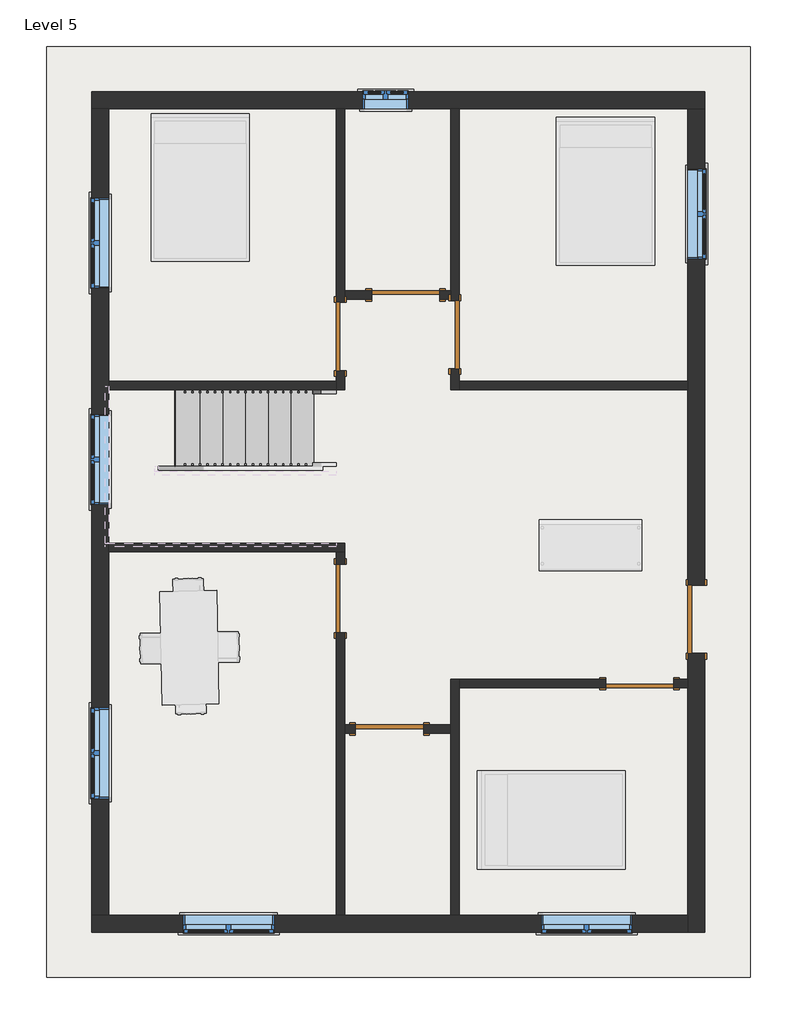
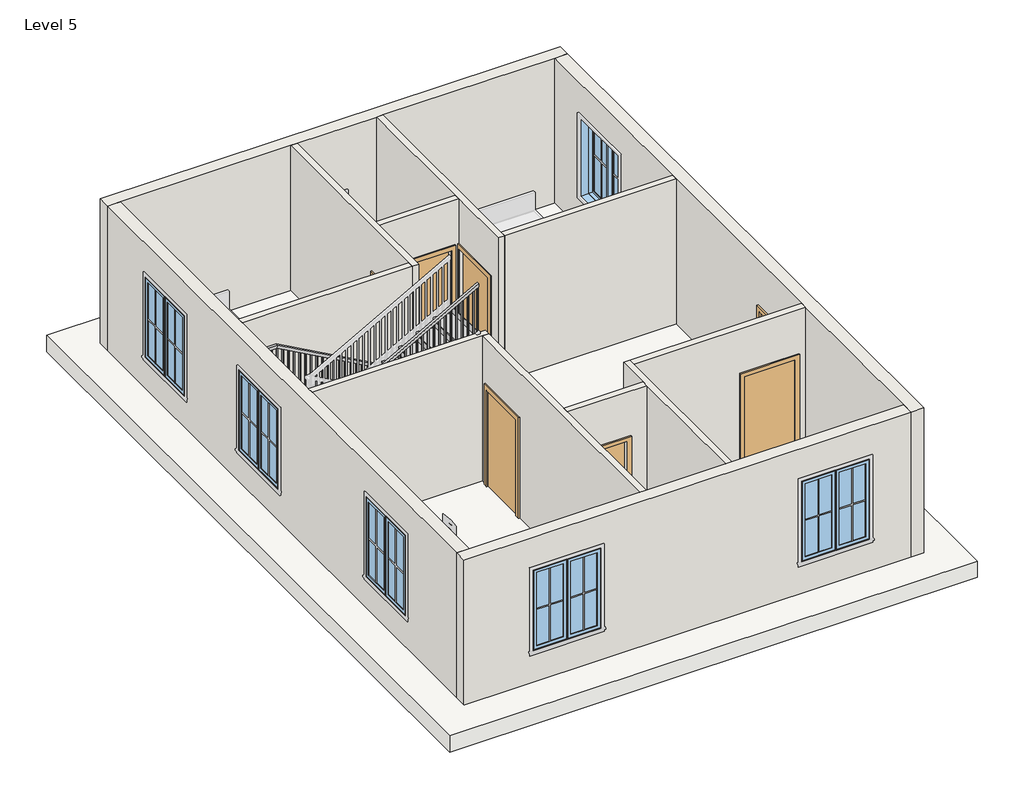
# One storey, part 1 of 2: 14 walls, 7 doors, 7 windows, 1 railing, 1 roof, 1 stair flight.
"""IFC4 building model written with IfcOpenShell, lengths in millimetres."""

from ifc_helpers import new_model, si_unit, frame, origin, place, context, project, spatial, polyline, outline, extrude, faceted_brep, transform, mapped, element, save
from components import door_e5f9f3c4, door_305aa2a5, door_a90ba1ad, stair_flight_99e02ff8, window_c417fced, window_8377141f

model = new_model("IFC4")

# Units and contexts
model_context = context("Model", 3, world=origin())
ifc_project = project(units=[si_unit("LENGTHUNIT", "METRE", prefix="MILLI")], contexts=[model_context])

# Site, building, storey
site = spatial("IfcSite", under=ifc_project)
building = spatial("IfcBuilding", under=site)
storey = spatial("IfcBuildingStorey", under=building, Name="Level 5", Elevation=12192.0)

# Doors
placement = place(None, origin())
door_shape = door_e5f9f3c4(model_context)
element("IfcDoor", 1, ObjectType="Single-Flush : 36\" x 84\"", at=placement, inside=storey, context=model_context, shape_type="MappedRepresentation", body=[
    mapped(door_shape, transform((5226.05, 11245.85, 12192.0), x_axis=(1.0, 0.0, 0.0), y_axis=(0.0, 1.0, 0.0), z_axis=(0.0, 0.0, 1.0))),
])
element("IfcDoor", 2, ObjectType="Single-Flush : 36\" x 84\"", at=placement, inside=storey, context=model_context, shape_type="MappedRepresentation", body=[
    mapped(door_shape, transform((5886.45, 10712.45, 12192.0), x_axis=(0.0, -1.0, 0.0), y_axis=(1.0, 0.0, 0.0), z_axis=(0.0, 0.0, 1.0))),
])
door_2_shape = door_305aa2a5(model_context)
element("IfcDoor", 3, ObjectType="Single-Flush : 36\" x 84\"", at=placement, inside=storey, context=model_context, shape_type="MappedRepresentation", body=[
    mapped(door_2_shape, transform((4349.75, 10687.05, 12192.0), x_axis=(0.0, -1.0, 0.0), y_axis=(1.0, 0.0, 0.0), z_axis=(0.0, 0.0, 1.0))),
])
element("IfcDoor", 4, ObjectType="Single-Flush : 36\" x 84\"", at=placement, inside=storey, context=model_context, shape_type="MappedRepresentation", body=[
    mapped(door_2_shape, transform((8369.3, 6026.15, 12192.0), x_axis=(1.0, 0.0, 0.0), y_axis=(0.0, 1.0, 0.0), z_axis=(0.0, 0.0, 1.0))),
])
element("IfcDoor", 5, ObjectType="Single-Flush : 36\" x 84\"", at=placement, inside=storey, context=model_context, shape_type="MappedRepresentation", body=[
    mapped(door_2_shape, transform((5010.15, 5416.55, 12192.0), x_axis=(-1.0, 0.0, 0.0), y_axis=(0.0, -1.0, 0.0), z_axis=(0.0, 0.0, 1.0))),
])
element("IfcDoor", 6, ObjectType="Single-Flush : 36\" x 84\"", at=placement, inside=storey, context=model_context, shape_type="MappedRepresentation", body=[
    mapped(door_2_shape, transform((4349.75, 7169.15, 12192.0), x_axis=(0.0, -1.0, 0.0), y_axis=(1.0, 0.0, 0.0), z_axis=(0.0, 0.0, 1.0))),
])
door_3_shape = door_a90ba1ad(model_context)
element("IfcDoor", 7, ObjectType="Single-Flush : 36\" x 84\"", at=placement, inside=storey, context=model_context, shape_type="MappedRepresentation", body=[
    mapped(door_3_shape, transform((9131.3, 6889.75, 12192.0), x_axis=(0.0, -1.0, 0.0), y_axis=(1.0, 0.0, 0.0), z_axis=(0.0, 0.0, 1.0))),
])

# Railing
element("IfcRailing", 8, ObjectType="Handrail - Rectangular", at=placement, inside=storey, context=model_context, shape_type="SolidModel", body=[
    faceted_brep([(4295.1355783, 9918.7, 13275.7333333), (4295.1355783, 9918.7, 13217.620221), (4295.1355783, 9969.5, 13217.620221), (4295.1355783, 9969.5, 13275.7333333), (1856.7355783, 9918.7, 14630.4), (1843.5719761, 9918.7, 14579.6), (1843.5719761, 9969.5, 14579.6), (1856.7355783, 9969.5, 14630.4), (1295.4, 9918.7, 14630.4), (1295.4, 9918.7, 14579.6), (1244.6, 9969.5, 14579.6), (1244.6, 9969.5, 14630.4), (1295.4, 7962.9, 14630.4), (1295.4, 7962.9, 14579.6), (1244.6, 7912.1, 14579.6), (1244.6, 7912.1, 14630.4), (1551.9355783, 7962.9, 14630.4), (1565.0991806, 7962.9, 14579.6), (1565.0991806, 7912.1, 14579.6), (1551.9355783, 7912.1, 14630.4), (4295.1355783, 7962.9, 16154.4), (4295.1355783, 7912.1, 16154.4), (4295.1355783, 7912.1, 16096.2868876), (4295.1355783, 7962.9, 16096.2868876)], [[[0, 1, 2, 3]], [[1, 0, 4, 5]], [[2, 1, 5, 6]], [[3, 2, 6, 7]], [[0, 3, 7, 4]], [[5, 4, 8, 9]], [[6, 5, 9, 10]], [[7, 6, 10, 11]], [[4, 7, 11, 8]], [[9, 8, 12, 13]], [[10, 9, 13, 14]], [[11, 10, 14, 15]], [[8, 11, 15, 12]], [[13, 12, 16, 17]], [[14, 13, 17, 18]], [[15, 14, 18, 19]], [[12, 15, 19, 16]], [[20, 21, 22, 23]], [[17, 16, 20, 23]], [[18, 17, 23, 22]], [[19, 18, 22, 21]], [[16, 19, 21, 20]]]),
    extrude(outline(polyline([(16057.8365664, 4225.925), (16047.253233, 4206.875), (15070.6666667, 4206.875), (15070.6666667, 4225.925), (16057.8365664, 4225.925)])), frame((0.0, 7927.975, 0.0), z_axis=(0.0, 1.0, 0.0), x_axis=(0.0, 0.0, 1.0)), (0.0, 0.0, 1.0), 19.05),
    extrude(outline(polyline([(16001.3921219, 4124.325), (15990.8087886, 4105.275), (15070.6666667, 4105.275), (15070.6666667, 4124.325), (16001.3921219, 4124.325)])), frame((0.0, 7927.975, 0.0), z_axis=(0.0, 1.0, 0.0), x_axis=(0.0, 0.0, 1.0)), (0.0, 0.0, 1.0), 19.05),
    extrude(outline(polyline([(15944.9476775, 4022.725), (15934.3643441, 4003.675), (15070.6666667, 4003.675), (15070.6666667, 4022.725), (15944.9476775, 4022.725)])), frame((0.0, 7927.975, 0.0), z_axis=(0.0, 1.0, 0.0), x_axis=(0.0, 0.0, 1.0)), (0.0, 0.0, 1.0), 19.05),
    extrude(outline(polyline([(15888.503233, 3921.125), (15877.9198997, 3902.075), (14901.3333333, 3902.075), (14901.3333333, 3921.125), (15888.503233, 3921.125)])), frame((0.0, 7927.975, 0.0), z_axis=(0.0, 1.0, 0.0), x_axis=(0.0, 0.0, 1.0)), (0.0, 0.0, 1.0), 19.05),
    extrude(outline(polyline([(15832.0587886, 3819.525), (15821.4754552, 3800.475), (14901.3333333, 3800.475), (14901.3333333, 3819.525), (15832.0587886, 3819.525)])), frame((0.0, 7927.975, 0.0), z_axis=(0.0, 1.0, 0.0), x_axis=(0.0, 0.0, 1.0)), (0.0, 0.0, 1.0), 19.05),
    extrude(outline(polyline([(15775.6143441, 3717.925), (15765.0310108, 3698.875), (14901.3333333, 3698.875), (14901.3333333, 3717.925), (15775.6143441, 3717.925)])), frame((0.0, 7927.975, 0.0), z_axis=(0.0, 1.0, 0.0), x_axis=(0.0, 0.0, 1.0)), (0.0, 0.0, 1.0), 19.05),
    extrude(outline(polyline([(15719.1698997, 3616.325), (15708.5865664, 3597.275), (14732.0, 3597.275), (14732.0, 3616.325), (15719.1698997, 3616.325)])), frame((0.0, 7927.975, 0.0), z_axis=(0.0, 1.0, 0.0), x_axis=(0.0, 0.0, 1.0)), (0.0, 0.0, 1.0), 19.05),
    extrude(outline(polyline([(15662.7254552, 3514.725), (15652.1421219, 3495.675), (14732.0, 3495.675), (14732.0, 3514.725), (15662.7254552, 3514.725)])), frame((0.0, 7927.975, 0.0), z_axis=(0.0, 1.0, 0.0), x_axis=(0.0, 0.0, 1.0)), (0.0, 0.0, 1.0), 19.05),
    extrude(outline(polyline([(15606.2810108, 3413.125), (15595.6976775, 3394.075), (14732.0, 3394.075), (14732.0, 3413.125), (15606.2810108, 3413.125)])), frame((0.0, 7927.975, 0.0), z_axis=(0.0, 1.0, 0.0), x_axis=(0.0, 0.0, 1.0)), (0.0, 0.0, 1.0), 19.05),
    extrude(outline(polyline([(15549.8365664, 3311.525), (15539.253233, 3292.475), (14562.6666667, 3292.475), (14562.6666667, 3311.525), (15549.8365664, 3311.525)])), frame((0.0, 7927.975, 0.0), z_axis=(0.0, 1.0, 0.0), x_axis=(0.0, 0.0, 1.0)), (0.0, 0.0, 1.0), 19.05),
    extrude(outline(polyline([(15493.3921219, 3209.925), (15482.8087886, 3190.875), (14562.6666667, 3190.875), (14562.6666667, 3209.925), (15493.3921219, 3209.925)])), frame((0.0, 7927.975, 0.0), z_axis=(0.0, 1.0, 0.0), x_axis=(0.0, 0.0, 1.0)), (0.0, 0.0, 1.0), 19.05),
    extrude(outline(polyline([(15436.9476775, 3108.325), (15426.3643441, 3089.275), (14562.6666667, 3089.275), (14562.6666667, 3108.325), (15436.9476775, 3108.325)])), frame((0.0, 7927.975, 0.0), z_axis=(0.0, 1.0, 0.0), x_axis=(0.0, 0.0, 1.0)), (0.0, 0.0, 1.0), 19.05),
    extrude(outline(polyline([(15380.503233, 3006.725), (15369.9198997, 2987.675), (14393.3333333, 2987.675), (14393.3333333, 3006.725), (15380.503233, 3006.725)])), frame((0.0, 7927.975, 0.0), z_axis=(0.0, 1.0, 0.0), x_axis=(0.0, 0.0, 1.0)), (0.0, 0.0, 1.0), 19.05),
    extrude(outline(polyline([(15324.0587886, 2905.125), (15313.4754552, 2886.075), (14393.3333333, 2886.075), (14393.3333333, 2905.125), (15324.0587886, 2905.125)])), frame((0.0, 7927.975, 0.0), z_axis=(0.0, 1.0, 0.0), x_axis=(0.0, 0.0, 1.0)), (0.0, 0.0, 1.0), 19.05),
    extrude(outline(polyline([(15267.6143441, 2803.525), (15257.0310108, 2784.475), (14393.3333333, 2784.475), (14393.3333333, 2803.525), (15267.6143441, 2803.525)])), frame((0.0, 7927.975, 0.0), z_axis=(0.0, 1.0, 0.0), x_axis=(0.0, 0.0, 1.0)), (0.0, 0.0, 1.0), 19.05),
    extrude(outline(polyline([(15211.1698997, 2701.925), (15200.5865664, 2682.875), (14224.0, 2682.875), (14224.0, 2701.925), (15211.1698997, 2701.925)])), frame((0.0, 7927.975, 0.0), z_axis=(0.0, 1.0, 0.0), x_axis=(0.0, 0.0, 1.0)), (0.0, 0.0, 1.0), 19.05),
    extrude(outline(polyline([(15154.7254552, 2600.325), (15144.1421219, 2581.275), (14224.0, 2581.275), (14224.0, 2600.325), (15154.7254552, 2600.325)])), frame((0.0, 7927.975, 0.0), z_axis=(0.0, 1.0, 0.0), x_axis=(0.0, 0.0, 1.0)), (0.0, 0.0, 1.0), 19.05),
    extrude(outline(polyline([(15098.2810108, 2498.725), (15087.6976775, 2479.675), (14224.0, 2479.675), (14224.0, 2498.725), (15098.2810108, 2498.725)])), frame((0.0, 7927.975, 0.0), z_axis=(0.0, 1.0, 0.0), x_axis=(0.0, 0.0, 1.0)), (0.0, 0.0, 1.0), 19.05),
    extrude(outline(polyline([(15041.8365664, 2397.125), (15031.253233, 2378.075), (14054.6666667, 2378.075), (14054.6666667, 2397.125), (15041.8365664, 2397.125)])), frame((0.0, 7927.975, 0.0), z_axis=(0.0, 1.0, 0.0), x_axis=(0.0, 0.0, 1.0)), (0.0, 0.0, 1.0), 19.05),
    extrude(outline(polyline([(14985.3921219, 2295.525), (14974.8087886, 2276.475), (14054.6666667, 2276.475), (14054.6666667, 2295.525), (14985.3921219, 2295.525)])), frame((0.0, 7927.975, 0.0), z_axis=(0.0, 1.0, 0.0), x_axis=(0.0, 0.0, 1.0)), (0.0, 0.0, 1.0), 19.05),
    extrude(outline(polyline([(14928.9476775, 2193.925), (14918.3643441, 2174.875), (14054.6666667, 2174.875), (14054.6666667, 2193.925), (14928.9476775, 2193.925)])), frame((0.0, 7927.975, 0.0), z_axis=(0.0, 1.0, 0.0), x_axis=(0.0, 0.0, 1.0)), (0.0, 0.0, 1.0), 19.05),
    extrude(outline(polyline([(14872.503233, 2092.325), (14861.9198997, 2073.275), (13885.3333333, 2073.275), (13885.3333333, 2092.325), (14872.503233, 2092.325)])), frame((0.0, 7927.975, 0.0), z_axis=(0.0, 1.0, 0.0), x_axis=(0.0, 0.0, 1.0)), (0.0, 0.0, 1.0), 19.05),
    extrude(outline(polyline([(14816.0587886, 1990.725), (14805.4754552, 1971.675), (13885.3333333, 1971.675), (13885.3333333, 1990.725), (14816.0587886, 1990.725)])), frame((0.0, 7927.975, 0.0), z_axis=(0.0, 1.0, 0.0), x_axis=(0.0, 0.0, 1.0)), (0.0, 0.0, 1.0), 19.05),
    extrude(outline(polyline([(14759.6143441, 1889.125), (14749.0310108, 1870.075), (13885.3333333, 1870.075), (13885.3333333, 1889.125), (14759.6143441, 1889.125)])), frame((0.0, 7927.975, 0.0), z_axis=(0.0, 1.0, 0.0), x_axis=(0.0, 0.0, 1.0)), (0.0, 0.0, 1.0), 19.05),
    extrude(outline(polyline([(14703.1698997, 1787.525), (14692.5865664, 1768.475), (13716.0, 1768.475), (13716.0, 1787.525), (14703.1698997, 1787.525)])), frame((0.0, 7927.975, 0.0), z_axis=(0.0, 1.0, 0.0), x_axis=(0.0, 0.0, 1.0)), (0.0, 0.0, 1.0), 19.05),
    extrude(outline(polyline([(14646.7254552, 1685.925), (14636.1421219, 1666.875), (13716.0, 1666.875), (13716.0, 1685.925), (14646.7254552, 1685.925)])), frame((0.0, 7927.975, 0.0), z_axis=(0.0, 1.0, 0.0), x_axis=(0.0, 0.0, 1.0)), (0.0, 0.0, 1.0), 19.05),
    extrude(outline(polyline([(14590.2810108, 1584.325), (14579.6976775, 1565.275), (13716.0, 1565.275), (13716.0, 1584.325), (14590.2810108, 1584.325)])), frame((0.0, 7927.975, 0.0), z_axis=(0.0, 1.0, 0.0), x_axis=(0.0, 0.0, 1.0)), (0.0, 0.0, 1.0), 19.05),
    extrude(outline(polyline([(1463.675, 7927.975), (1463.675, 7947.025), (1482.725, 7947.025), (1482.725, 7927.975), (1463.675, 7927.975)])), frame((0.0, 0.0, 13716.0), z_axis=(0.0, 0.0, 1.0), x_axis=(1.0, 0.0, 0.0)), (0.0, 0.0, 1.0), 863.6),
    extrude(outline(polyline([(1362.075, 7927.975), (1362.075, 7947.025), (1381.125, 7947.025), (1381.125, 7927.975), (1362.075, 7927.975)])), frame((0.0, 0.0, 13716.0), z_axis=(0.0, 0.0, 1.0), x_axis=(1.0, 0.0, 0.0)), (0.0, 0.0, 1.0), 863.6),
    extrude(outline(polyline([(1260.475, 8023.225), (1279.525, 8023.225), (1279.525, 8004.175), (1260.475, 8004.175), (1260.475, 8023.225)])), frame((0.0, 0.0, 13716.0), z_axis=(0.0, 0.0, 1.0), x_axis=(1.0, 0.0, 0.0)), (0.0, 0.0, 1.0), 863.6),
    extrude(outline(polyline([(1260.475, 8124.825), (1279.525, 8124.825), (1279.525, 8105.775), (1260.475, 8105.775), (1260.475, 8124.825)])), frame((0.0, 0.0, 13716.0), z_axis=(0.0, 0.0, 1.0), x_axis=(1.0, 0.0, 0.0)), (0.0, 0.0, 1.0), 863.6),
    extrude(outline(polyline([(1260.475, 8226.425), (1279.525, 8226.425), (1279.525, 8207.375), (1260.475, 8207.375), (1260.475, 8226.425)])), frame((0.0, 0.0, 13716.0), z_axis=(0.0, 0.0, 1.0), x_axis=(1.0, 0.0, 0.0)), (0.0, 0.0, 1.0), 863.6),
    extrude(outline(polyline([(1260.475, 8328.025), (1279.525, 8328.025), (1279.525, 8308.975), (1260.475, 8308.975), (1260.475, 8328.025)])), frame((0.0, 0.0, 13716.0), z_axis=(0.0, 0.0, 1.0), x_axis=(1.0, 0.0, 0.0)), (0.0, 0.0, 1.0), 863.6),
    extrude(outline(polyline([(1260.475, 8429.625), (1279.525, 8429.625), (1279.525, 8410.575), (1260.475, 8410.575), (1260.475, 8429.625)])), frame((0.0, 0.0, 13716.0), z_axis=(0.0, 0.0, 1.0), x_axis=(1.0, 0.0, 0.0)), (0.0, 0.0, 1.0), 863.6),
    extrude(outline(polyline([(1260.475, 8531.225), (1279.525, 8531.225), (1279.525, 8512.175), (1260.475, 8512.175), (1260.475, 8531.225)])), frame((0.0, 0.0, 13716.0), z_axis=(0.0, 0.0, 1.0), x_axis=(1.0, 0.0, 0.0)), (0.0, 0.0, 1.0), 863.6),
    extrude(outline(polyline([(1260.475, 8632.825), (1279.525, 8632.825), (1279.525, 8613.775), (1260.475, 8613.775), (1260.475, 8632.825)])), frame((0.0, 0.0, 13716.0), z_axis=(0.0, 0.0, 1.0), x_axis=(1.0, 0.0, 0.0)), (0.0, 0.0, 1.0), 863.6),
    extrude(outline(polyline([(1260.475, 8734.425), (1279.525, 8734.425), (1279.525, 8715.375), (1260.475, 8715.375), (1260.475, 8734.425)])), frame((0.0, 0.0, 13716.0), z_axis=(0.0, 0.0, 1.0), x_axis=(1.0, 0.0, 0.0)), (0.0, 0.0, 1.0), 863.6),
    extrude(outline(polyline([(1260.475, 8836.025), (1279.525, 8836.025), (1279.525, 8816.975), (1260.475, 8816.975), (1260.475, 8836.025)])), frame((0.0, 0.0, 13716.0), z_axis=(0.0, 0.0, 1.0), x_axis=(1.0, 0.0, 0.0)), (0.0, 0.0, 1.0), 863.6),
    extrude(outline(polyline([(1260.475, 8937.625), (1279.525, 8937.625), (1279.525, 8918.575), (1260.475, 8918.575), (1260.475, 8937.625)])), frame((0.0, 0.0, 13716.0), z_axis=(0.0, 0.0, 1.0), x_axis=(1.0, 0.0, 0.0)), (0.0, 0.0, 1.0), 863.6),
    extrude(outline(polyline([(1260.475, 9039.225), (1279.525, 9039.225), (1279.525, 9020.175), (1260.475, 9020.175), (1260.475, 9039.225)])), frame((0.0, 0.0, 13716.0), z_axis=(0.0, 0.0, 1.0), x_axis=(1.0, 0.0, 0.0)), (0.0, 0.0, 1.0), 863.6),
    extrude(outline(polyline([(1260.475, 9140.825), (1279.525, 9140.825), (1279.525, 9121.775), (1260.475, 9121.775), (1260.475, 9140.825)])), frame((0.0, 0.0, 13716.0), z_axis=(0.0, 0.0, 1.0), x_axis=(1.0, 0.0, 0.0)), (0.0, 0.0, 1.0), 863.6),
    extrude(outline(polyline([(1260.475, 9242.425), (1279.525, 9242.425), (1279.525, 9223.375), (1260.475, 9223.375), (1260.475, 9242.425)])), frame((0.0, 0.0, 13716.0), z_axis=(0.0, 0.0, 1.0), x_axis=(1.0, 0.0, 0.0)), (0.0, 0.0, 1.0), 863.6),
    extrude(outline(polyline([(1260.475, 9344.025), (1279.525, 9344.025), (1279.525, 9324.975), (1260.475, 9324.975), (1260.475, 9344.025)])), frame((0.0, 0.0, 13716.0), z_axis=(0.0, 0.0, 1.0), x_axis=(1.0, 0.0, 0.0)), (0.0, 0.0, 1.0), 863.6),
    extrude(outline(polyline([(1260.475, 9445.625), (1279.525, 9445.625), (1279.525, 9426.575), (1260.475, 9426.575), (1260.475, 9445.625)])), frame((0.0, 0.0, 13716.0), z_axis=(0.0, 0.0, 1.0), x_axis=(1.0, 0.0, 0.0)), (0.0, 0.0, 1.0), 863.6),
    extrude(outline(polyline([(1260.475, 9547.225), (1279.525, 9547.225), (1279.525, 9528.175), (1260.475, 9528.175), (1260.475, 9547.225)])), frame((0.0, 0.0, 13716.0), z_axis=(0.0, 0.0, 1.0), x_axis=(1.0, 0.0, 0.0)), (0.0, 0.0, 1.0), 863.6),
    extrude(outline(polyline([(1260.475, 9648.825), (1279.525, 9648.825), (1279.525, 9629.775), (1260.475, 9629.775), (1260.475, 9648.825)])), frame((0.0, 0.0, 13716.0), z_axis=(0.0, 0.0, 1.0), x_axis=(1.0, 0.0, 0.0)), (0.0, 0.0, 1.0), 863.6),
    extrude(outline(polyline([(1260.475, 9750.425), (1279.525, 9750.425), (1279.525, 9731.375), (1260.475, 9731.375), (1260.475, 9750.425)])), frame((0.0, 0.0, 13716.0), z_axis=(0.0, 0.0, 1.0), x_axis=(1.0, 0.0, 0.0)), (0.0, 0.0, 1.0), 863.6),
    extrude(outline(polyline([(1260.475, 9852.025), (1279.525, 9852.025), (1279.525, 9832.975), (1260.475, 9832.975), (1260.475, 9852.025)])), frame((0.0, 0.0, 13716.0), z_axis=(0.0, 0.0, 1.0), x_axis=(1.0, 0.0, 0.0)), (0.0, 0.0, 1.0), 863.6),
    extrude(outline(polyline([(1358.2605783, 9953.625), (1358.2605783, 9934.575), (1339.2105783, 9934.575), (1339.2105783, 9953.625), (1358.2605783, 9953.625)])), frame((0.0, 0.0, 13716.0), z_axis=(0.0, 0.0, 1.0), x_axis=(1.0, 0.0, 0.0)), (0.0, 0.0, 1.0), 863.6),
    extrude(outline(polyline([(1459.8605783, 9953.625), (1459.8605783, 9934.575), (1440.8105783, 9934.575), (1440.8105783, 9953.625), (1459.8605783, 9953.625)])), frame((0.0, 0.0, 13716.0), z_axis=(0.0, 0.0, 1.0), x_axis=(1.0, 0.0, 0.0)), (0.0, 0.0, 1.0), 863.6),
    extrude(outline(polyline([(1561.4605783, 9953.625), (1561.4605783, 9934.575), (1542.4105783, 9934.575), (1542.4105783, 9953.625), (1561.4605783, 9953.625)])), frame((0.0, 0.0, 13716.0), z_axis=(0.0, 0.0, 1.0), x_axis=(1.0, 0.0, 0.0)), (0.0, 0.0, 1.0), 863.6),
    extrude(outline(polyline([(1663.0605783, 9953.625), (1663.0605783, 9934.575), (1644.0105783, 9934.575), (1644.0105783, 9953.625), (1663.0605783, 9953.625)])), frame((0.0, 0.0, 13716.0), z_axis=(0.0, 0.0, 1.0), x_axis=(1.0, 0.0, 0.0)), (0.0, 0.0, 1.0), 863.6),
    extrude(outline(polyline([(1764.6605783, 9953.625), (1764.6605783, 9934.575), (1745.6105783, 9934.575), (1745.6105783, 9953.625), (1764.6605783, 9953.625)])), frame((0.0, 0.0, 13716.0), z_axis=(0.0, 0.0, 1.0), x_axis=(1.0, 0.0, 0.0)), (0.0, 0.0, 1.0), 863.6),
    extrude(outline(polyline([(14566.995221, 1866.2605783), (14577.5785543, 1847.2105783), (13716.0, 1847.2105783), (13716.0, 1866.2605783), (14566.995221, 1866.2605783)])), frame((0.0, 9934.575, 0.0), z_axis=(0.0, 1.0, 0.0), x_axis=(0.0, 0.0, 1.0)), (0.0, 0.0, 1.0), 19.05),
    extrude(outline(polyline([(14510.5507765, 1967.8605783), (14521.1341099, 1948.8105783), (13546.6666667, 1948.8105783), (13546.6666667, 1967.8605783), (14510.5507765, 1967.8605783)])), frame((0.0, 9934.575, 0.0), z_axis=(0.0, 1.0, 0.0), x_axis=(0.0, 0.0, 1.0)), (0.0, 0.0, 1.0), 19.05),
    extrude(outline(polyline([(14454.1063321, 2069.4605783), (14464.6896654, 2050.4105783), (13546.6666667, 2050.4105783), (13546.6666667, 2069.4605783), (14454.1063321, 2069.4605783)])), frame((0.0, 9934.575, 0.0), z_axis=(0.0, 1.0, 0.0), x_axis=(0.0, 0.0, 1.0)), (0.0, 0.0, 1.0), 19.05),
    extrude(outline(polyline([(14397.6618876, 2171.0605783), (14408.245221, 2152.0105783), (13546.6666667, 2152.0105783), (13546.6666667, 2171.0605783), (14397.6618876, 2171.0605783)])), frame((0.0, 9934.575, 0.0), z_axis=(0.0, 1.0, 0.0), x_axis=(0.0, 0.0, 1.0)), (0.0, 0.0, 1.0), 19.05),
    extrude(outline(polyline([(14341.2174432, 2272.6605783), (14351.8007765, 2253.6105783), (13377.3333333, 2253.6105783), (13377.3333333, 2272.6605783), (14341.2174432, 2272.6605783)])), frame((0.0, 9934.575, 0.0), z_axis=(0.0, 1.0, 0.0), x_axis=(0.0, 0.0, 1.0)), (0.0, 0.0, 1.0), 19.05),
    extrude(outline(polyline([(14284.7729988, 2374.2605783), (14295.3563321, 2355.2105783), (13377.3333333, 2355.2105783), (13377.3333333, 2374.2605783), (14284.7729988, 2374.2605783)])), frame((0.0, 9934.575, 0.0), z_axis=(0.0, 1.0, 0.0), x_axis=(0.0, 0.0, 1.0)), (0.0, 0.0, 1.0), 19.05),
    extrude(outline(polyline([(14228.3285543, 2475.8605783), (14238.9118876, 2456.8105783), (13377.3333333, 2456.8105783), (13377.3333333, 2475.8605783), (14228.3285543, 2475.8605783)])), frame((0.0, 9934.575, 0.0), z_axis=(0.0, 1.0, 0.0), x_axis=(0.0, 0.0, 1.0)), (0.0, 0.0, 1.0), 19.05),
    extrude(outline(polyline([(14171.8841099, 2577.4605783), (14182.4674432, 2558.4105783), (13208.0, 2558.4105783), (13208.0, 2577.4605783), (14171.8841099, 2577.4605783)])), frame((0.0, 9934.575, 0.0), z_axis=(0.0, 1.0, 0.0), x_axis=(0.0, 0.0, 1.0)), (0.0, 0.0, 1.0), 19.05),
    extrude(outline(polyline([(14115.4396654, 2679.0605783), (14126.0229988, 2660.0105783), (13208.0, 2660.0105783), (13208.0, 2679.0605783), (14115.4396654, 2679.0605783)])), frame((0.0, 9934.575, 0.0), z_axis=(0.0, 1.0, 0.0), x_axis=(0.0, 0.0, 1.0)), (0.0, 0.0, 1.0), 19.05),
    extrude(outline(polyline([(14058.995221, 2780.6605783), (14069.5785543, 2761.6105783), (13208.0, 2761.6105783), (13208.0, 2780.6605783), (14058.995221, 2780.6605783)])), frame((0.0, 9934.575, 0.0), z_axis=(0.0, 1.0, 0.0), x_axis=(0.0, 0.0, 1.0)), (0.0, 0.0, 1.0), 19.05),
    extrude(outline(polyline([(14002.5507765, 2882.2605783), (14013.1341099, 2863.2105783), (13038.6666667, 2863.2105783), (13038.6666667, 2882.2605783), (14002.5507765, 2882.2605783)])), frame((0.0, 9934.575, 0.0), z_axis=(0.0, 1.0, 0.0), x_axis=(0.0, 0.0, 1.0)), (0.0, 0.0, 1.0), 19.05),
    extrude(outline(polyline([(13946.1063321, 2983.8605783), (13956.6896654, 2964.8105783), (13038.6666667, 2964.8105783), (13038.6666667, 2983.8605783), (13946.1063321, 2983.8605783)])), frame((0.0, 9934.575, 0.0), z_axis=(0.0, 1.0, 0.0), x_axis=(0.0, 0.0, 1.0)), (0.0, 0.0, 1.0), 19.05),
    extrude(outline(polyline([(13889.6618876, 3085.4605783), (13900.245221, 3066.4105783), (13038.6666667, 3066.4105783), (13038.6666667, 3085.4605783), (13889.6618876, 3085.4605783)])), frame((0.0, 9934.575, 0.0), z_axis=(0.0, 1.0, 0.0), x_axis=(0.0, 0.0, 1.0)), (0.0, 0.0, 1.0), 19.05),
    extrude(outline(polyline([(13833.2174432, 3187.0605783), (13843.8007765, 3168.0105783), (12869.3333333, 3168.0105783), (12869.3333333, 3187.0605783), (13833.2174432, 3187.0605783)])), frame((0.0, 9934.575, 0.0), z_axis=(0.0, 1.0, 0.0), x_axis=(0.0, 0.0, 1.0)), (0.0, 0.0, 1.0), 19.05),
    extrude(outline(polyline([(13776.7729988, 3288.6605783), (13787.3563321, 3269.6105783), (12869.3333333, 3269.6105783), (12869.3333333, 3288.6605783), (13776.7729988, 3288.6605783)])), frame((0.0, 9934.575, 0.0), z_axis=(0.0, 1.0, 0.0), x_axis=(0.0, 0.0, 1.0)), (0.0, 0.0, 1.0), 19.05),
    extrude(outline(polyline([(13720.3285543, 3390.2605783), (13730.9118876, 3371.2105783), (12869.3333333, 3371.2105783), (12869.3333333, 3390.2605783), (13720.3285543, 3390.2605783)])), frame((0.0, 9934.575, 0.0), z_axis=(0.0, 1.0, 0.0), x_axis=(0.0, 0.0, 1.0)), (0.0, 0.0, 1.0), 19.05),
    extrude(outline(polyline([(13663.8841099, 3491.8605783), (13674.4674432, 3472.8105783), (12700.0, 3472.8105783), (12700.0, 3491.8605783), (13663.8841099, 3491.8605783)])), frame((0.0, 9934.575, 0.0), z_axis=(0.0, 1.0, 0.0), x_axis=(0.0, 0.0, 1.0)), (0.0, 0.0, 1.0), 19.05),
    extrude(outline(polyline([(13607.4396654, 3593.4605783), (13618.0229988, 3574.4105783), (12700.0, 3574.4105783), (12700.0, 3593.4605783), (13607.4396654, 3593.4605783)])), frame((0.0, 9934.575, 0.0), z_axis=(0.0, 1.0, 0.0), x_axis=(0.0, 0.0, 1.0)), (0.0, 0.0, 1.0), 19.05),
    extrude(outline(polyline([(13550.995221, 3695.0605783), (13561.5785543, 3676.0105783), (12700.0, 3676.0105783), (12700.0, 3695.0605783), (13550.995221, 3695.0605783)])), frame((0.0, 9934.575, 0.0), z_axis=(0.0, 1.0, 0.0), x_axis=(0.0, 0.0, 1.0)), (0.0, 0.0, 1.0), 19.05),
    extrude(outline(polyline([(13494.5507765, 3796.6605783), (13505.1341099, 3777.6105783), (12530.6666667, 3777.6105783), (12530.6666667, 3796.6605783), (13494.5507765, 3796.6605783)])), frame((0.0, 9934.575, 0.0), z_axis=(0.0, 1.0, 0.0), x_axis=(0.0, 0.0, 1.0)), (0.0, 0.0, 1.0), 19.05),
    extrude(outline(polyline([(13438.1063321, 3898.2605783), (13448.6896654, 3879.2105783), (12530.6666667, 3879.2105783), (12530.6666667, 3898.2605783), (13438.1063321, 3898.2605783)])), frame((0.0, 9934.575, 0.0), z_axis=(0.0, 1.0, 0.0), x_axis=(0.0, 0.0, 1.0)), (0.0, 0.0, 1.0), 19.05),
    extrude(outline(polyline([(13381.6618876, 3999.8605783), (13392.245221, 3980.8105783), (12530.6666667, 3980.8105783), (12530.6666667, 3999.8605783), (13381.6618876, 3999.8605783)])), frame((0.0, 9934.575, 0.0), z_axis=(0.0, 1.0, 0.0), x_axis=(0.0, 0.0, 1.0)), (0.0, 0.0, 1.0), 19.05),
    extrude(outline(polyline([(13325.2174432, 4101.4605783), (13335.8007765, 4082.4105783), (12361.3333333, 4082.4105783), (12361.3333333, 4101.4605783), (13325.2174432, 4101.4605783)])), frame((0.0, 9934.575, 0.0), z_axis=(0.0, 1.0, 0.0), x_axis=(0.0, 0.0, 1.0)), (0.0, 0.0, 1.0), 19.05),
    extrude(outline(polyline([(13268.7729988, 4203.0605783), (13279.3563321, 4184.0105783), (12361.3333333, 4184.0105783), (12361.3333333, 4203.0605783), (13268.7729988, 4203.0605783)])), frame((0.0, 9934.575, 0.0), z_axis=(0.0, 1.0, 0.0), x_axis=(0.0, 0.0, 1.0)), (0.0, 0.0, 1.0), 19.05),
    extrude(outline(polyline([(1260.475, 7947.025), (1279.525, 7947.025), (1279.525, 7927.975), (1260.475, 7927.975), (1260.475, 7947.025)])), frame((0.0, 0.0, 13716.0), z_axis=(0.0, 0.0, 1.0), x_axis=(1.0, 0.0, 0.0)), (0.0, 0.0, 1.0), 863.6),
    extrude(outline(polyline([(1279.525, 9953.625), (1279.525, 9934.575), (1260.475, 9934.575), (1260.475, 9953.625), (1279.525, 9953.625)])), frame((0.0, 0.0, 13716.0), z_axis=(0.0, 0.0, 1.0), x_axis=(1.0, 0.0, 0.0)), (0.0, 0.0, 1.0), 863.6),
    extrude(outline(polyline([(16096.2868876, 4295.1355783), (16085.7035543, 4276.0855783), (15070.6666667, 4276.0855783), (15070.6666667, 4295.1355783), (16096.2868876, 4295.1355783)])), frame((0.0, 7927.975, 0.0), z_axis=(0.0, 1.0, 0.0), x_axis=(0.0, 0.0, 1.0)), (0.0, 0.0, 1.0), 19.05),
    extrude(outline(polyline([(13217.620221, 4295.1355783), (13228.2035543, 4276.0855783), (12361.3333333, 4276.0855783), (12361.3333333, 4295.1355783), (13217.620221, 4295.1355783)])), frame((0.0, 9934.575, 0.0), z_axis=(0.0, 1.0, 0.0), x_axis=(0.0, 0.0, 1.0)), (0.0, 0.0, 1.0), 19.05),
])

# Roof
element("IfcRoof", 9, ObjectType="Generic - 12\"", at=placement, inside=storey, context=model_context, shape_type="SweptSolid", body=[
    extrude(outline(polyline([(406.4, 14579.6), (9855.2, 14579.6), (9855.2, 2082.8), (406.4, 2082.8), (406.4, 14579.6)])), frame((0.0, 0.0, 12192.0), z_axis=(0.0, 0.0, 1.0), x_axis=(1.0, 0.0, 0.0)), (0.0, 0.0, 1.0), 304.8),
])

# Stair flight
stair_flight_shape = stair_flight_99e02ff8(model_context)
element("IfcStairFlight", 10, ObjectType="2\" Tread 1\" Nosing 1/4\" Riser", at=placement, inside=storey, context=model_context, shape_type="MappedRepresentation", body=[
    mapped(stair_flight_shape, transform((0.0, 0.0, 0.0), x_axis=(1.0, 0.0, 0.0), y_axis=(0.0, 1.0, 0.0), z_axis=(0.0, 0.0, 1.0))),
])

# Walls
element("IfcWall", 11, ObjectType="Generic - 5\"", at=placement, inside=storey, context=model_context, shape_type="Brep", body=[
    faceted_brep([(4292.6, 10229.85, 14325.6), (4292.6, 10229.85, 12192.0), (4292.6, 10083.8, 12192.0), (4292.6, 9969.5, 12192.0), (4292.6, 9969.5, 15240.0), (4292.6, 10083.8, 15240.0), (4292.6, 13741.4, 15240.0), (4292.6, 13741.4, 12192.0), (4292.6, 11144.25, 12192.0), (4292.6, 11144.25, 14325.6), (4406.9, 9969.5, 12192.0), (4406.9, 10229.85, 12192.0), (4406.9, 10229.85, 14325.6), (4406.9, 11144.25, 14325.6), (4406.9, 11144.25, 12192.0), (4406.9, 11188.7, 12192.0), (4406.9, 11303.0, 12192.0), (4406.9, 13741.4, 12192.0), (4406.9, 13741.4, 15240.0), (4406.9, 11303.0, 15240.0), (4406.9, 11188.7, 15240.0), (4406.9, 9969.5, 15240.0)], [[[0, 1, 2, 3, 4, 5, 6, 7, 8, 9]], [[10, 11, 12, 13, 14, 15, 16, 17, 18, 19, 20, 21]], [[8, 7, 17, 16, 15, 14]], [[3, 2, 1, 11, 10]], [[6, 5, 4, 21, 20, 19, 18]], [[7, 6, 18, 17]], [[4, 3, 10, 21]], [[12, 11, 1, 0]], [[13, 12, 0, 9]], [[14, 13, 9, 8]]]),
])
element("IfcWall", 12, ObjectType="Generic - 5\"", at=placement, inside=storey, context=model_context, shape_type="SweptSolid", body=[
    extrude(outline(polyline([(1244.6, 10083.8), (4292.6, 10083.8), (4292.6, 9969.5), (1244.6, 9969.5), (1244.6, 10083.8)])), frame((0.0, 0.0, 12192.0), z_axis=(0.0, 0.0, 1.0), x_axis=(1.0, 0.0, 0.0)), (0.0, 0.0, 1.0), 3048.0),
])
element("IfcWall", 13, ObjectType="Generic - 5\"", at=placement, inside=storey, context=model_context, shape_type="SweptSolid", body=[
    extrude(outline(polyline([(14325.6, 5683.25), (12192.0, 5683.25), (12192.0, 5829.3), (15240.0, 5829.3), (15240.0, 4406.9), (12192.0, 4406.9), (12192.0, 4768.85), (14325.6, 4768.85), (14325.6, 5683.25)])), frame((0.0, 11188.7, 0.0), z_axis=(0.0, 1.0, 0.0), x_axis=(0.0, 0.0, 1.0)), (0.0, 0.0, 1.0), 114.3),
])
element("IfcWall", 14, ObjectType="Generic - 5\"", at=placement, inside=storey, context=model_context, shape_type="Brep", body=[
    faceted_brep([(5829.3, 10255.25, 14325.6), (5829.3, 10255.25, 12192.0), (5829.3, 9969.5, 12192.0), (5829.3, 9969.5, 15240.0), (5829.3, 11188.7, 15240.0), (5829.3, 11303.0, 15240.0), (5829.3, 13741.4, 15240.0), (5829.3, 13741.4, 12192.0), (5829.3, 11303.0, 12192.0), (5829.3, 11188.7, 12192.0), (5829.3, 11169.65, 12192.0), (5829.3, 11169.65, 14325.6), (5943.6, 9969.5, 12192.0), (5943.6, 10083.8, 12192.0), (5943.6, 10255.25, 12192.0), (5943.6, 10255.25, 14325.6), (5943.6, 11169.65, 14325.6), (5943.6, 11169.65, 12192.0), (5943.6, 13741.4, 12192.0), (5943.6, 13741.4, 15240.0), (5943.6, 10083.8, 15240.0), (5943.6, 9969.5, 15240.0)], [[[0, 1, 2, 3, 4, 5, 6, 7, 8, 9, 10, 11]], [[12, 13, 14, 15, 16, 17, 18, 19, 20, 21]], [[2, 1, 14, 13, 12]], [[10, 9, 8, 7, 18, 17]], [[6, 5, 4, 3, 21, 20, 19]], [[7, 6, 19, 18]], [[3, 2, 12, 21]], [[15, 14, 1, 0]], [[16, 15, 0, 11]], [[17, 16, 11, 10]]]),
])
element("IfcWall", 15, ObjectType="Generic - 5\"", at=placement, inside=storey, context=model_context, shape_type="SweptSolid", body=[
    extrude(outline(polyline([(9017.0, 9969.5), (5943.6, 9969.5), (5943.6, 10083.8), (9017.0, 10083.8), (9017.0, 9969.5)])), frame((0.0, 0.0, 12192.0), z_axis=(0.0, 0.0, 1.0), x_axis=(1.0, 0.0, 0.0)), (0.0, 0.0, 1.0), 3048.0),
])
element("IfcWall", 16, ObjectType="Generic - 5\"", at=placement, inside=storey, context=model_context, shape_type="Brep", body=[
    faceted_brep([(1244.6, 7797.8, 12192.0), (4292.6, 7797.8, 12192.0), (4406.9, 7797.8, 12192.0), (4406.9, 7797.8, 15240.0), (4292.6, 7797.8, 15240.0), (1244.6, 7797.8, 15240.0), (1244.6, 7912.1, 12192.0), (1244.6, 7912.1, 15240.0), (4406.9, 7912.1, 15240.0), (4406.9, 7912.1, 12192.0)], [[[0, 1, 2, 3, 4, 5]], [[6, 7, 8, 9]], [[2, 1, 0, 6, 9]], [[5, 4, 3, 8, 7]], [[0, 5, 7, 6]], [[3, 2, 9, 8]]]),
])
element("IfcWall", 17, ObjectType="Generic - 5\"", at=placement, inside=storey, context=model_context, shape_type="Brep", body=[
    faceted_brep([(4292.6, 6711.95, 14325.6), (4292.6, 6711.95, 12192.0), (4292.6, 2921.0, 12192.0), (4292.6, 2921.0, 15240.0), (4292.6, 7797.8, 15240.0), (4292.6, 7797.8, 12192.0), (4292.6, 7626.35, 12192.0), (4292.6, 7626.35, 14325.6), (4406.9, 2921.0, 12192.0), (4406.9, 5359.4, 12192.0), (4406.9, 5473.7, 12192.0), (4406.9, 6711.95, 12192.0), (4406.9, 6711.95, 14325.6), (4406.9, 7626.35, 14325.6), (4406.9, 7626.35, 12192.0), (4406.9, 7797.8, 12192.0), (4406.9, 7797.8, 15240.0), (4406.9, 5473.7, 15240.0), (4406.9, 5359.4, 15240.0), (4406.9, 2921.0, 15240.0)], [[[0, 1, 2, 3, 4, 5, 6, 7]], [[8, 9, 10, 11, 12, 13, 14, 15, 16, 17, 18, 19]], [[6, 5, 15, 14]], [[2, 1, 11, 10, 9, 8]], [[4, 3, 19, 18, 17, 16]], [[5, 4, 16, 15]], [[3, 2, 8, 19]], [[12, 11, 1, 0]], [[13, 12, 0, 7]], [[14, 13, 7, 6]]]),
])
element("IfcWall", 18, ObjectType="Generic - 5\"", at=placement, inside=storey, context=model_context, shape_type="SweptSolid", body=[
    extrude(outline(polyline([(12192.0, 4406.9), (12192.0, 4552.95), (14325.6, 4552.95), (14325.6, 5467.35), (12192.0, 5467.35), (12192.0, 5829.3), (15240.0, 5829.3), (15240.0, 4406.9), (12192.0, 4406.9)])), frame((0.0, 5359.4, 0.0), z_axis=(0.0, 1.0, 0.0), x_axis=(0.0, 0.0, 1.0)), (0.0, 0.0, 1.0), 114.3),
])
element("IfcWall", 19, ObjectType="Generic - 5\"", at=placement, inside=storey, context=model_context, shape_type="Brep", body=[
    faceted_brep([(5943.6, 2921.0, 12192.0), (5943.6, 5969.0, 12192.0), (5943.6, 6083.3, 12192.0), (5943.6, 6083.3, 15240.0), (5943.6, 5969.0, 15240.0), (5943.6, 2921.0, 15240.0), (5829.3, 2921.0, 12192.0), (5829.3, 2921.0, 15240.0), (5829.3, 5359.4, 15240.0), (5829.3, 5473.7, 15240.0), (5829.3, 6083.3, 15240.0), (5829.3, 6083.3, 12192.0), (5829.3, 5473.7, 12192.0), (5829.3, 5359.4, 12192.0)], [[[0, 1, 2, 3, 4, 5]], [[6, 7, 8, 9, 10, 11, 12, 13]], [[2, 1, 0, 6, 13, 12, 11]], [[5, 4, 3, 10, 9, 8, 7]], [[0, 5, 7, 6]], [[3, 2, 11, 10]]]),
])
element("IfcWall", 20, ObjectType="Generic - 5\"", at=placement, inside=storey, context=model_context, shape_type="SweptSolid", body=[
    extrude(outline(polyline([(14325.6, 8826.5), (12192.0, 8826.5), (12192.0, 9017.0), (15240.0, 9017.0), (15240.0, 5943.6), (12192.0, 5943.6), (12192.0, 7912.1), (14325.6, 7912.1), (14325.6, 8826.5)])), frame((0.0, 5969.0, 0.0), z_axis=(0.0, 1.0, 0.0), x_axis=(0.0, 0.0, 1.0)), (0.0, 0.0, 1.0), 114.3),
])
element("IfcWall", 21, ObjectType="Generic - 8\"", at=placement, inside=storey, context=model_context, shape_type="Brep", body=[
    faceted_brep([(1016.0, 13741.4, 12192.0), (1244.6, 13741.4, 12192.0), (4292.6, 13741.4, 12192.0), (4406.9, 13741.4, 12192.0), (5829.3, 13741.4, 12192.0), (5943.6, 13741.4, 12192.0), (9017.0, 13741.4, 12192.0), (9245.6, 13741.4, 12192.0), (9245.6, 13741.4, 15240.0), (9017.0, 13741.4, 15240.0), (5943.6, 13741.4, 15240.0), (5829.3, 13741.4, 15240.0), (4406.9, 13741.4, 15240.0), (4292.6, 13741.4, 15240.0), (1244.6, 13741.4, 15240.0), (1016.0, 13741.4, 15240.0), (5264.15, 13741.4, 14020.8), (5264.15, 13741.4, 13106.4), (4654.55, 13741.4, 13106.4), (4654.55, 13741.4, 14020.8), (1016.0, 13970.0, 12192.0), (1016.0, 13970.0, 15240.0), (9245.6, 13970.0, 15240.0), (9245.6, 13970.0, 12192.0), (5264.15, 13970.0, 14020.8), (4654.55, 13970.0, 14020.8), (4654.55, 13970.0, 13106.4), (5264.15, 13970.0, 13106.4)], [[[0, 1, 2, 3, 4, 5, 6, 7, 8, 9, 10, 11, 12, 13, 14, 15], [16, 17, 18, 19]], [[20, 21, 22, 23], [24, 25, 26, 27]], [[7, 6, 5, 4, 3, 2, 1, 0, 20, 23]], [[15, 14, 13, 12, 11, 10, 9, 8, 22, 21]], [[8, 7, 23, 22]], [[0, 15, 21, 20]], [[17, 16, 24, 27]], [[18, 17, 27, 26]], [[19, 18, 26, 25]], [[16, 19, 25, 24]]]),
])
element("IfcWall", 22, ObjectType="Generic - 8\"", at=placement, inside=storey, context=model_context, shape_type="Brep", body=[
    faceted_brep([(9017.0, 6432.55, 14325.6), (9017.0, 6432.55, 12192.0), (9017.0, 6083.3, 12192.0), (9017.0, 5969.0, 12192.0), (9017.0, 2921.0, 12192.0), (9017.0, 2692.4, 12192.0), (9017.0, 2692.4, 15240.0), (9017.0, 2921.0, 15240.0), (9017.0, 5969.0, 15240.0), (9017.0, 6083.3, 15240.0), (9017.0, 9969.5, 15240.0), (9017.0, 10083.8, 15240.0), (9017.0, 13741.4, 15240.0), (9017.0, 13741.4, 12192.0), (9017.0, 10083.8, 12192.0), (9017.0, 9969.5, 12192.0), (9017.0, 7346.95, 12192.0), (9017.0, 7346.95, 14325.6), (9017.0, 11722.1, 14630.4), (9017.0, 11722.1, 13106.4), (9017.0, 12941.3, 13106.4), (9017.0, 12941.3, 14630.4), (9245.6, 2692.4, 12192.0), (9245.6, 6432.55, 12192.0), (9245.6, 6432.55, 14325.6), (9245.6, 7346.95, 14325.6), (9245.6, 7346.95, 12192.0), (9245.6, 13741.4, 12192.0), (9245.6, 13741.4, 15240.0), (9245.6, 2692.4, 15240.0), (9245.6, 11722.1, 14630.4), (9245.6, 12941.3, 14630.4), (9245.6, 12941.3, 13106.4), (9245.6, 11722.1, 13106.4)], [[[0, 1, 2, 3, 4, 5, 6, 7, 8, 9, 10, 11, 12, 13, 14, 15, 16, 17], [18, 19, 20, 21]], [[22, 23, 24, 25, 26, 27, 28, 29], [30, 31, 32, 33]], [[5, 4, 3, 2, 1, 23, 22]], [[16, 15, 14, 13, 27, 26]], [[12, 11, 10, 9, 8, 7, 6, 29, 28]], [[13, 12, 28, 27]], [[6, 5, 22, 29]], [[24, 23, 1, 0]], [[25, 24, 0, 17]], [[26, 25, 17, 16]], [[19, 18, 30, 33]], [[20, 19, 33, 32]], [[21, 20, 32, 31]], [[18, 21, 31, 30]]]),
])
element("IfcWall", 23, ObjectType="Generic - 8\"", at=placement, inside=storey, context=model_context, shape_type="Brep", body=[
    faceted_brep([(9017.0, 2921.0, 12192.0), (5943.6, 2921.0, 12192.0), (5829.3, 2921.0, 12192.0), (4406.9, 2921.0, 12192.0), (4292.6, 2921.0, 12192.0), (1244.6, 2921.0, 12192.0), (1016.0, 2921.0, 12192.0), (1016.0, 2921.0, 15240.0), (1244.6, 2921.0, 15240.0), (4292.6, 2921.0, 15240.0), (4406.9, 2921.0, 15240.0), (5829.3, 2921.0, 15240.0), (5943.6, 2921.0, 15240.0), (9017.0, 2921.0, 15240.0), (7048.5, 2921.0, 14630.4), (7048.5, 2921.0, 13106.4), (8267.7, 2921.0, 13106.4), (8267.7, 2921.0, 14630.4), (2241.55, 2921.0, 14630.4), (2241.55, 2921.0, 13106.4), (3460.75, 2921.0, 13106.4), (3460.75, 2921.0, 14630.4), (9017.0, 2692.4, 12192.0), (9017.0, 2692.4, 15240.0), (1016.0, 2692.4, 15240.0), (1016.0, 2692.4, 12192.0), (7048.5, 2692.4, 14630.4), (8267.7, 2692.4, 14630.4), (8267.7, 2692.4, 13106.4), (7048.5, 2692.4, 13106.4), (2241.55, 2692.4, 14630.4), (3460.75, 2692.4, 14630.4), (3460.75, 2692.4, 13106.4), (2241.55, 2692.4, 13106.4)], [[[0, 1, 2, 3, 4, 5, 6, 7, 8, 9, 10, 11, 12, 13], [14, 15, 16, 17], [18, 19, 20, 21]], [[22, 23, 24, 25], [26, 27, 28, 29], [30, 31, 32, 33]], [[6, 5, 4, 3, 2, 1, 0, 22, 25]], [[13, 12, 11, 10, 9, 8, 7, 24, 23]], [[0, 13, 23, 22]], [[7, 6, 25, 24]], [[15, 14, 26, 29]], [[16, 15, 29, 28]], [[17, 16, 28, 27]], [[14, 17, 27, 26]], [[19, 18, 30, 33]], [[20, 19, 33, 32]], [[21, 20, 32, 31]], [[18, 21, 31, 30]]]),
])
element("IfcWall", 24, ObjectType="Generic - 8\"", at=placement, inside=storey, context=model_context, shape_type="Brep", body=[
    faceted_brep([(1244.6, 2921.0, 12192.0), (1244.6, 7797.8, 12192.0), (1244.6, 7912.1, 12192.0), (1244.6, 9969.5, 12192.0), (1244.6, 10083.8, 12192.0), (1244.6, 13741.4, 12192.0), (1244.6, 13741.4, 15240.0), (1244.6, 10083.8, 15240.0), (1244.6, 9969.5, 15240.0), (1244.6, 7912.1, 15240.0), (1244.6, 7797.8, 15240.0), (1244.6, 2921.0, 15240.0), (1244.6, 5702.3, 14630.4), (1244.6, 5702.3, 13106.4), (1244.6, 4483.1, 13106.4), (1244.6, 4483.1, 14630.4), (1244.6, 9645.65, 14630.4), (1244.6, 9645.65, 13106.4), (1244.6, 8426.45, 13106.4), (1244.6, 8426.45, 14630.4), (1244.6, 12550.775, 14630.4), (1244.6, 12550.775, 13106.4), (1244.6, 11331.575, 13106.4), (1244.6, 11331.575, 14630.4), (1016.0, 2921.0, 12192.0), (1016.0, 2921.0, 15240.0), (1016.0, 13741.4, 15240.0), (1016.0, 13741.4, 12192.0), (1016.0, 5702.3, 14630.4), (1016.0, 4483.1, 14630.4), (1016.0, 4483.1, 13106.4), (1016.0, 5702.3, 13106.4), (1016.0, 9645.65, 14630.4), (1016.0, 8426.45, 14630.4), (1016.0, 8426.45, 13106.4), (1016.0, 9645.65, 13106.4), (1016.0, 12550.775, 14630.4), (1016.0, 11331.575, 14630.4), (1016.0, 11331.575, 13106.4), (1016.0, 12550.775, 13106.4)], [[[0, 1, 2, 3, 4, 5, 6, 7, 8, 9, 10, 11], [12, 13, 14, 15], [16, 17, 18, 19], [20, 21, 22, 23]], [[24, 25, 26, 27], [28, 29, 30, 31], [32, 33, 34, 35], [36, 37, 38, 39]], [[5, 4, 3, 2, 1, 0, 24, 27]], [[11, 10, 9, 8, 7, 6, 26, 25]], [[6, 5, 27, 26]], [[0, 11, 25, 24]], [[13, 12, 28, 31]], [[14, 13, 31, 30]], [[15, 14, 30, 29]], [[12, 15, 29, 28]], [[17, 16, 32, 35]], [[18, 17, 35, 34]], [[19, 18, 34, 33]], [[16, 19, 33, 32]], [[21, 20, 36, 39]], [[22, 21, 39, 38]], [[23, 22, 38, 37]], [[20, 23, 37, 36]]]),
])

# Windows
window_shape = window_c417fced(model_context)
element("IfcWindow", 25, ObjectType="Window-Casement-Double : 24\" x 36\"", at=placement, inside=storey, context=model_context, shape_type="MappedRepresentation", body=[
    mapped(window_shape, transform((4959.35, 13855.7, 12192.0), x_axis=(1.0, 0.0, 0.0), y_axis=(0.0, 1.0, 0.0), z_axis=(0.0, 0.0, 1.0))),
])
window_2_shape = window_8377141f(model_context)
element("IfcWindow", 26, ObjectType="Window-Casement-Double : 48\" x 60\"", at=placement, inside=storey, context=model_context, shape_type="MappedRepresentation", body=[
    mapped(window_2_shape, transform((7658.1, 2806.7, 12192.0), x_axis=(-1.0, 0.0, 0.0), y_axis=(0.0, -1.0, 0.0), z_axis=(0.0, 0.0, 1.0))),
])
element("IfcWindow", 27, ObjectType="Window-Casement-Double : 48\" x 60\"", at=placement, inside=storey, context=model_context, shape_type="MappedRepresentation", body=[
    mapped(window_2_shape, transform((2851.15, 2806.7, 12192.0), x_axis=(-1.0, 0.0, 0.0), y_axis=(0.0, -1.0, 0.0), z_axis=(0.0, 0.0, 1.0))),
])
element("IfcWindow", 28, ObjectType="Window-Casement-Double : 48\" x 60\"", at=placement, inside=storey, context=model_context, shape_type="MappedRepresentation", body=[
    mapped(window_2_shape, transform((1130.3, 5092.7, 12192.0), x_axis=(0.0, 1.0, 0.0), y_axis=(-1.0, 0.0, 0.0), z_axis=(0.0, 0.0, 1.0))),
])
element("IfcWindow", 29, ObjectType="Window-Casement-Double : 48\" x 60\"", at=placement, inside=storey, context=model_context, shape_type="MappedRepresentation", body=[
    mapped(window_2_shape, transform((1130.3, 9036.05, 12192.0), x_axis=(0.0, 1.0, 0.0), y_axis=(-1.0, 0.0, 0.0), z_axis=(0.0, 0.0, 1.0))),
])
element("IfcWindow", 30, ObjectType="Window-Casement-Double : 48\" x 60\"", at=placement, inside=storey, context=model_context, shape_type="MappedRepresentation", body=[
    mapped(window_2_shape, transform((1130.3, 11941.175, 12192.0), x_axis=(0.0, 1.0, 0.0), y_axis=(-1.0, 0.0, 0.0), z_axis=(0.0, 0.0, 1.0))),
])
element("IfcWindow", 31, ObjectType="Window-Casement-Double : 48\" x 60\"", at=placement, inside=storey, context=model_context, shape_type="MappedRepresentation", body=[
    mapped(window_2_shape, transform((9131.3, 12331.7, 12192.0), x_axis=(0.0, -1.0, 0.0), y_axis=(1.0, 0.0, 0.0), z_axis=(0.0, 0.0, 1.0))),
])

save(model, "model.ifc")

# Revit data of these elements
# Type "Single-Flush : 36\" x 84\""
#   Type Mark = "1"
#   Construction Type Id = "MDOOR"
#   Assembly Code = "C1020"
#   Analytic Construction = "Metal"
#   Thickness = 0' - 2"
#   Heat Transfer Coefficient (U) = 0.651978 BTU/(h·ft²·°F)
#   Height = 7' - 0"
#   Trim Projection Ext = 0' - 1"
#   Trim Projection Int = 0' - 1"
#   Trim Width = 0' - 3"
#   Width = 3' - 0"
#   Define Thermal Properties by = 1
#   Define Thermal Properties by = 1
#   Door Material = Door - Panel
#   Frame Material = Door - Frame
#   Visual Light Transmittance = 0
#   Solar Heat Gain Coefficient = 0
#   Function = (empty or 0)
#   Wall Closure = (empty or 0)
# Type "Handrail - Rectangular"
#   Assembly Code = "C2010400"
#   built-in parameter 1008612 = 0.0416667 (stored number, unit not read)
#   built-in parameter 1008611 = 0.0416667 (stored number, unit not read)
#   built-in parameter 1008609 = 0.333333 (stored number, unit not read)
#   built-in parameter 1008604 = 0.166667 (stored number, unit not read)
#   built-in parameter 1008603 = 0.166667 (stored number, unit not read)
#   Railing Height = 3' - 0"
#   built-in parameter 1008630 = 2
#   built-in parameter 1008610 = 2
#   built-in parameter 1008618 = Baluster - Square : 3/4"
# Type "Generic - 12\""
#   Assembly Code = "B1020"
#   Layers, outside or top first: 1' - 0" no material (function 1)
# Type "Generic - 5\""
#   Assembly Code = "B2010"
#   Layers, outside or top first: 0' - 4 1/2" no material (function 1)
# Type "Generic - 8\""
#   Assembly Code = "B2010"
#   Layers, outside or top first: 0' - 9" no material (function 1)
# Type "Window-Casement-Double : 24\" x 36\""
#   Type Mark = "14"
#   Fire Rating = "0.5h"
#   Assembly Code = "B2020100"
#   Analytic Construction = "Double glazing - domestic"
#   Frame Extension [instance default] = 0' - 0 1/4"
#   Window Inset [instance default] = 0' - 0"
#   Wall Thickness [instance default] = 0' - 6"
#   Interior Wall Closure [instance default] = 0' - 2 1/4"
#   Half Width = 1' - 0"
#   Visual Light Transmittance = 0.81
#   Thermal Resistance (R) = 1.8146 (h·ft²·°F)/BTU
#   Solar Heat Gain Coefficient = 0.76
#   Rough Width = 2' - 0 1/2"
#   Rough Height = 3' - 0 1/2"
#   Height = 3' - 0"
#   Heat Transfer Coefficient (U) = 0.5511 BTU/(h·ft²·°F)
#   Exterior Wall Closure [instance default] = 0' - 1 1/4"
#   Extension Jamb [instance default] = 0' - 2 1/4"
#   Default Sill Height = 3' - 0"
#   Width = 2' - 0"
#   Define Thermal Properties by = 0
#   Muntin Visibility = yes
#   Interior Trim Visibility [instance default] = yes
#   Exterior Trim Visibility [instance default] = yes
#   Extension Jamb Visibility [instance default] = yes
#   Interior Trim Material = Wood - Stained
#   Muntin Pattern = Muntin Pattern_2x2 : Muntin Pattern_2x2
#   Interior Trim = Trim-Window-Interior-Flat : Picture Frame
#   Interior Frame Material = Wood - Stained
#   Glass Panel Material = Glass
#   Exterior Trim Material = Clad - White
#   Exterior Trim = Trim-Window-Exterior-Flat : with Sill
#   Exterior Frame Material = Clad - White
#   Wall Closure = (empty or 0)
# Type "Window-Casement-Double : 48\" x 60\""
#   Type Mark = "17"
#   Fire Rating = "0.5h"
#   Assembly Code = "B2020100"
#   Analytic Construction = "Double glazing - domestic"
#   Frame Extension [instance default] = 0' - 0 1/4"
#   Window Inset [instance default] = 0' - 0"
#   Wall Thickness [instance default] = 0' - 6"
#   Interior Wall Closure [instance default] = 0' - 2 1/4"
#   Half Width = 2' - 0"
#   Visual Light Transmittance = 0.81
#   Thermal Resistance (R) = 1.8146 (h·ft²·°F)/BTU
#   Solar Heat Gain Coefficient = 0.76
#   Rough Width = 4' - 0 1/2"
#   Rough Height = 5' - 0 1/2"
#   Height = 5' - 0"
#   Heat Transfer Coefficient (U) = 0.5511 BTU/(h·ft²·°F)
#   Exterior Wall Closure [instance default] = 0' - 1 1/4"
#   Extension Jamb [instance default] = 0' - 2 1/4"
#   Default Sill Height = 3' - 0"
#   Width = 4' - 0"
#   Define Thermal Properties by = 0
#   Muntin Visibility = yes
#   Interior Trim Visibility [instance default] = yes
#   Exterior Trim Visibility [instance default] = yes
#   Extension Jamb Visibility [instance default] = yes
#   Interior Trim Material = Wood - Stained
#   Muntin Pattern = Muntin Pattern_2x2 : Muntin Pattern_2x2
#   Interior Trim = Trim-Window-Interior-Flat : Picture Frame
#   Interior Frame Material = Wood - Stained
#   Glass Panel Material = Glass
#   Exterior Trim Material = Clad - White
#   Exterior Trim = Trim-Window-Exterior-Flat : with Sill
#   Exterior Frame Material = Clad - White
#   Wall Closure = (empty or 0)
# Elements 1, 2, 3, 4, 5, 6, 7 (IfcDoor, "Single-Flush : 36\" x 84\"")
#   Phase Created = New Construction
#   Materials on its faces: "Door - Frame", "Door - Panel"
# Element 8 (IfcRailing, "Handrail - Rectangular")
#   Phase Created = New Construction
# Element 9 (IfcRoof, "Generic - 12\"")
#   built-in parameter 1001705 = 41 (stored number, unit not read)
#   built-in parameter 1001710 = 33615
#   Phase Created = New Construction
#   Materials on its faces: "Flor_Branco", "Default Roof"
# Element 10 (IfcStairFlight, "2\" Tread 1\" Nosing 1/4\" Riser")
#   Phase Created = New Construction
# Elements 11, 12, 13, 14, 15, 16, 17, 18, 19, 20 (IfcWall, "Generic - 5\"")
#   Top Offset = 0' - 0"
#   Base Offset = 0' - 0"
#   wall height = 10' - 0"
#   Phase Created = New Construction
#   Base Constraint = Level 5
#   Top Constraint = Level 6
#   Materials on its faces: "Default Wall"
# Elements 21, 22, 23, 24 (IfcWall, "Generic - 8\"")
#   Top Offset = 0' - 0"
#   Base Offset = 0' - 0"
#   Unconnected Height = 10' - 0"
#   wall height = 10' - 0"
#   Phase Created = New Construction
#   Base Constraint = Level 5
#   Materials on its faces: "Default Wall", "Sash"
# Element 25 (IfcWindow, "Window-Casement-Double : 24\" x 36\"")
#   Mark = "35"
#   Window Inset = 0' - 0"
#   Interior Wall Closure = 0' - 2 1/4"
#   Frame Extension = 0' - 0 1/4"
#   Exterior Wall Closure = 0' - 1 1/4"
#   Interior Trim Visibility = yes
#   Exterior Trim Visibility = yes
#   Phase Created = New Construction
#   Materials on its faces: "Wood - Stained", "Glass", "Clad - White"
# Element 26 (IfcWindow, "Window-Casement-Double : 48\" x 60\"")
#   Mark = "29"
#   Window Inset = 0' - 0"
#   Interior Wall Closure = 0' - 2 1/4"
#   Frame Extension = 0' - 0 1/4"
#   Exterior Wall Closure = 0' - 1 1/4"
#   Interior Trim Visibility = yes
#   Exterior Trim Visibility = yes
#   Phase Created = New Construction
#   Materials on its faces: "Wood - Stained", "Glass", "Clad - White"
# Element 27 (IfcWindow, "Window-Casement-Double : 48\" x 60\"")
#   Mark = "30"
#   Window Inset = 0' - 0"
#   Interior Wall Closure = 0' - 2 1/4"
#   Frame Extension = 0' - 0 1/4"
#   Exterior Wall Closure = 0' - 1 1/4"
#   Interior Trim Visibility = yes
#   Exterior Trim Visibility = yes
#   Phase Created = New Construction
#   Materials on its faces: "Wood - Stained", "Glass", "Clad - White"
# Element 28 (IfcWindow, "Window-Casement-Double : 48\" x 60\"")
#   Mark = "31"
#   Window Inset = 0' - 0"
#   Interior Wall Closure = 0' - 2 1/4"
#   Frame Extension = 0' - 0 1/4"
#   Exterior Wall Closure = 0' - 1 1/4"
#   Interior Trim Visibility = yes
#   Exterior Trim Visibility = yes
#   Phase Created = New Construction
#   Materials on its faces: "Wood - Stained", "Glass", "Clad - White"
# Element 29 (IfcWindow, "Window-Casement-Double : 48\" x 60\"")
#   Mark = "32"
#   Window Inset = 0' - 0"
#   Interior Wall Closure = 0' - 2 1/4"
#   Frame Extension = 0' - 0 1/4"
#   Exterior Wall Closure = 0' - 1 1/4"
#   Interior Trim Visibility = yes
#   Exterior Trim Visibility = yes
#   Phase Created = New Construction
#   Materials on its faces: "Wood - Stained", "Glass", "Clad - White"
# Element 30 (IfcWindow, "Window-Casement-Double : 48\" x 60\"")
#   Mark = "33"
#   Window Inset = 0' - 0"
#   Interior Wall Closure = 0' - 2 1/4"
#   Frame Extension = 0' - 0 1/4"
#   Exterior Wall Closure = 0' - 1 1/4"
#   Interior Trim Visibility = yes
#   Exterior Trim Visibility = yes
#   Phase Created = New Construction
#   Materials on its faces: "Wood - Stained", "Glass", "Clad - White"
# Element 31 (IfcWindow, "Window-Casement-Double : 48\" x 60\"")
#   Mark = "34"
#   Window Inset = 0' - 0"
#   Interior Wall Closure = 0' - 2 1/4"
#   Frame Extension = 0' - 0 1/4"
#   Exterior Wall Closure = 0' - 1 1/4"
#   Interior Trim Visibility = yes
#   Exterior Trim Visibility = yes
